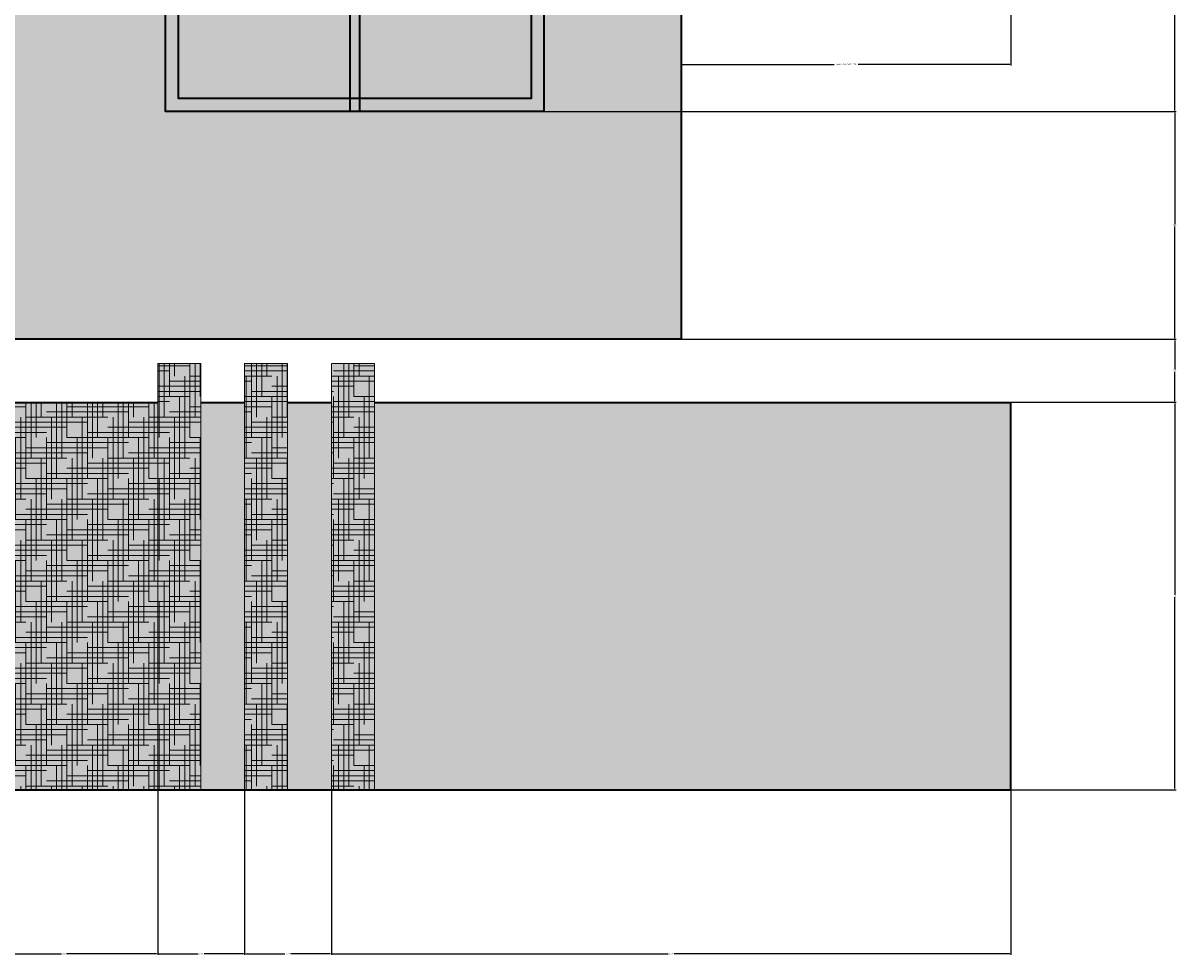
# Model space of a CAD drawing. Units: feet. Extents: x 2415 to 6174, y 866 to 1295.
# Tile 4 of 9: x 3580 to 3759, y 866 to 1010. Entities that reach past the tile are written whole.
import ezdxf

# ---------------------------------------------------------------- set-up
doc = ezdxf.new("R2010")
doc.units = ezdxf.units.FT
for name, color, linetype, lineweight in [('A-ANNO-DIMS', 2, 'Continuous', 18), ('A-ELEV', 7, 'Continuous', 35), ('A-ELEV-LOUV', 9, 'Continuous', 18), ('A-ELEV-PATT', 8, 'Continuous', 13)]:
    doc.layers.add(name, color=color, linetype=linetype, lineweight=lineweight)
doc.styles.get("Standard").update_dxf_attribs({"font": 'arial.ttf'})
doc.dimstyles.get("Standard").update_dxf_attribs({"dimtxt": 0.18, "dimasz": 0.18, "dimexe": 0.18, "dimexo": 0.0625, "dimgap": 0.09, "dimtad": 0, "dimtih": 1, "dimtoh": 1, "dimdec": 1, "dimzin": 0, "dimdsep": 46, "dimlunit": 3, "dimtxsty": 'Standard', "dimcen": 0.09, "dimadec": 0, "dimazin": 0, "dimtfac": 1, "dimtdec": 1, "dimtofl": 0, "dimtmove": 0, "dimatfit": 3, "dimfxl": 1, "dimtolj": 1, "dimtzin": 0, "dimarcsym": 0})

# ---------------------------------------------------------------- blocks, each defined once
blk = doc.blocks.new('FACADE-FIN')
blk.add_line((0, 66), (6.66, 66))
for points in [[(0, 0), (0, 66)], [(6.66, 66), (6.66, 0)]]:
    blk.add_lwpolyline(points)
blk = doc.blocks.new('*D13')
at = {"layer": 'A-ANNO-DIMS', "color": 0, "lineweight": -2, "transparency": 16777216}
for p, q in [((3682.07, 1011.54), (3682.07, 1003.76)), ((3733.13, 1011.54), (3733.13, 1003.76)), ((3682.25, 1003.94), (3705.76, 1003.94)), ((3732.95, 1003.94), (3709.45, 1003.94))]:
    blk.add_line(p, q, dxfattribs=at)
at = {"layer": 'A-ANNO-DIMS', "color": 0, "transparency": 16777216}
for points in [[(3682.25, 1003.97), (3682.25, 1003.91), (3682.07, 1003.94)], [(3732.95, 1003.97), (3732.95, 1003.91), (3733.13, 1003.94)]]:
    blk.add_solid(points, dxfattribs=at)
at = {"layer": 'Defpoints', "color": 0, "transparency": 16777216}
for p in [(3682.07, 1011.6), (3733.13, 1011.6), (3733.13, 1003.94)]:
    blk.add_point(p, dxfattribs=at)
at = {"layer": 'A-ANNO-DIMS', "color": 0, "transparency": 16777216, "insert": (3707.6, 1003.94), "char_height": 0.18, "attachment_point": 5}
blk.add_mtext('\\A1;BALCONY RAIL BASE 51 TYP.', dxfattribs=at)
blk = doc.blocks.new('*D57')
at = {"layer": 'A-ANNO-DIMS', "color": 0, "lineweight": -2, "transparency": 16777216}
for p, q in [((3571.93, 891.54), (3571.93, 866.02)), ((3601, 891.54), (3601, 866.02)), ((3572.11, 866.2), (3586.07, 866.2)), ((3600.82, 866.2), (3586.86, 866.2))]:
    blk.add_line(p, q, dxfattribs=at)
at = {"layer": 'A-ANNO-DIMS', "color": 0, "transparency": 16777216}
for points in [[(3572.11, 866.23), (3572.11, 866.17), (3571.93, 866.2)], [(3600.82, 866.23), (3600.82, 866.17), (3601, 866.2)]]:
    blk.add_solid(points, dxfattribs=at)
at = {"layer": 'Defpoints', "color": 0, "transparency": 16777216}
for p in [(3571.93, 891.6), (3601, 891.6), (3601, 866.2)]:
    blk.add_point(p, dxfattribs=at)
at = {"layer": 'A-ANNO-DIMS', "color": 0, "transparency": 16777216, "insert": (3586.47, 866.2), "char_height": 0.18, "attachment_point": 5}
blk.add_mtext('\\A1;29.06', dxfattribs=at)
blk = doc.blocks.new('*D58')
at = {"layer": 'A-ANNO-DIMS', "color": 0, "lineweight": -2, "transparency": 16777216}
for p, q in [((3601, 891.54), (3601, 866.02)), ((3614.44, 891.54), (3614.44, 866.02)), ((3601.18, 866.2), (3607.26, 866.2)), ((3614.26, 866.2), (3608.17, 866.2))]:
    blk.add_line(p, q, dxfattribs=at)
at = {"layer": 'A-ANNO-DIMS', "color": 0, "transparency": 16777216}
for points in [[(3601.18, 866.23), (3601.18, 866.17), (3601, 866.2)], [(3614.26, 866.23), (3614.26, 866.17), (3614.44, 866.2)]]:
    blk.add_solid(points, dxfattribs=at)
at = {"layer": 'Defpoints', "color": 0, "transparency": 16777216}
for p in [(3601, 891.6), (3614.44, 891.6), (3614.44, 866.2)]:
    blk.add_point(p, dxfattribs=at)
at = {"layer": 'A-ANNO-DIMS', "color": 0, "transparency": 16777216, "insert": (3607.72, 866.2), "char_height": 0.18, "attachment_point": 5}
blk.add_mtext('\\A1;13.442', dxfattribs=at)
blk = doc.blocks.new('*D59')
at = {"layer": 'A-ANNO-DIMS', "color": 0, "lineweight": -2, "transparency": 16777216}
for p, q in [((3614.44, 891.54), (3614.44, 866.02)), ((3627.88, 891.54), (3627.88, 866.02)), ((3614.62, 866.2), (3620.7, 866.2)), ((3627.7, 866.2), (3621.61, 866.2))]:
    blk.add_line(p, q, dxfattribs=at)
at = {"layer": 'A-ANNO-DIMS', "color": 0, "transparency": 16777216}
for points in [[(3614.62, 866.23), (3614.62, 866.17), (3614.44, 866.2)], [(3627.7, 866.23), (3627.7, 866.17), (3627.88, 866.2)]]:
    blk.add_solid(points, dxfattribs=at)
at = {"layer": 'Defpoints', "color": 0, "transparency": 16777216}
for p in [(3614.44, 891.6), (3627.88, 891.6), (3627.88, 866.2)]:
    blk.add_point(p, dxfattribs=at)
at = {"layer": 'A-ANNO-DIMS', "color": 0, "transparency": 16777216, "insert": (3621.16, 866.2), "char_height": 0.18, "attachment_point": 5}
blk.add_mtext('\\A1;13.442', dxfattribs=at)
blk = doc.blocks.new('*D60')
at = {"layer": 'A-ANNO-DIMS', "color": 0, "lineweight": -2, "transparency": 16777216}
for p, q in [((3627.88, 891.54), (3627.88, 866.02)), ((3733.13, 891.54), (3733.13, 866.02)), ((3628.06, 866.2), (3680.05, 866.2)), ((3732.95, 866.2), (3680.96, 866.2))]:
    blk.add_line(p, q, dxfattribs=at)
at = {"layer": 'A-ANNO-DIMS', "color": 0, "transparency": 16777216}
for points in [[(3628.06, 866.23), (3628.06, 866.17), (3627.88, 866.2)], [(3732.95, 866.23), (3732.95, 866.17), (3733.13, 866.2)]]:
    blk.add_solid(points, dxfattribs=at)
at = {"layer": 'Defpoints', "color": 0, "transparency": 16777216}
for p in [(3627.88, 891.6), (3733.13, 891.6), (3733.13, 866.2)]:
    blk.add_point(p, dxfattribs=at)
at = {"layer": 'A-ANNO-DIMS', "color": 0, "transparency": 16777216, "insert": (3680.5, 866.2), "char_height": 0.18, "attachment_point": 5}
blk.add_mtext('\\A1;105.25', dxfattribs=at)
blk = doc.blocks.new('*D79')
at = {"layer": 'A-ANNO-DIMS', "color": 0, "lineweight": -2, "transparency": 16777216}
for p, q in [((3733.19, 951.6), (3758.71, 951.6)), ((3758.53, 951.42), (3758.53, 921.78)), ((3758.53, 891.78), (3758.53, 921.42)), ((3733.19, 891.6), (3758.71, 891.6))]:
    blk.add_line(p, q, dxfattribs=at)
at = {"layer": 'A-ANNO-DIMS', "color": 0, "transparency": 16777216}
for points in [[(3758.5, 951.42), (3758.56, 951.42), (3758.53, 951.6)], [(3758.5, 891.78), (3758.56, 891.78), (3758.53, 891.6)]]:
    blk.add_solid(points, dxfattribs=at)
at = {"layer": 'Defpoints', "color": 0, "transparency": 16777216}
for p in [(3733.13, 951.6), (3758.53, 951.6), (3733.13, 891.6)]:
    blk.add_point(p, dxfattribs=at)
at = {"layer": 'A-ANNO-DIMS', "color": 0, "transparency": 16777216, "insert": (3758.53, 921.6), "char_height": 0.18, "attachment_point": 5}
blk.add_mtext('\\A1;60', dxfattribs=at)
blk = doc.blocks.new('*D80')
at = {"layer": 'A-ANNO-DIMS', "color": 0, "lineweight": -2, "transparency": 16777216}
for p, q in [((3682.13, 961.37), (3758.71, 961.37)), ((3758.53, 961.19), (3758.53, 956.66)), ((3758.53, 951.78), (3758.53, 956.3)), ((3733.19, 951.6), (3758.71, 951.6))]:
    blk.add_line(p, q, dxfattribs=at)
at = {"layer": 'A-ANNO-DIMS', "color": 0, "transparency": 16777216}
for points in [[(3758.5, 961.19), (3758.56, 961.19), (3758.53, 961.37)], [(3758.5, 951.78), (3758.56, 951.78), (3758.53, 951.6)]]:
    blk.add_solid(points, dxfattribs=at)
at = {"layer": 'Defpoints', "color": 0, "transparency": 16777216}
for p in [(3682.07, 961.37), (3758.53, 961.37), (3733.13, 951.6)]:
    blk.add_point(p, dxfattribs=at)
at = {"layer": 'A-ANNO-DIMS', "color": 0, "transparency": 16777216, "insert": (3758.53, 956.48), "char_height": 0.18, "attachment_point": 5}
blk.add_mtext('\\A1;9.766', dxfattribs=at)
blk = doc.blocks.new('*D81')
at = {"layer": 'A-ANNO-DIMS', "color": 0, "lineweight": -2, "transparency": 16777216}
for p, q in [((3660.88, 996.64), (3758.71, 996.64)), ((3758.53, 996.46), (3758.53, 979.19)), ((3758.53, 961.55), (3758.53, 978.82)), ((3682.13, 961.37), (3758.71, 961.37))]:
    blk.add_line(p, q, dxfattribs=at)
at = {"layer": 'A-ANNO-DIMS', "color": 0, "transparency": 16777216}
for points in [[(3758.5, 996.46), (3758.56, 996.46), (3758.53, 996.64)], [(3758.5, 961.55), (3758.56, 961.55), (3758.53, 961.37)]]:
    blk.add_solid(points, dxfattribs=at)
at = {"layer": 'Defpoints', "color": 0, "transparency": 16777216}
for p in [(3660.81, 996.64), (3758.53, 996.64), (3682.07, 961.37)]:
    blk.add_point(p, dxfattribs=at)
at = {"layer": 'A-ANNO-DIMS', "color": 0, "transparency": 16777216, "insert": (3758.53, 979.01), "char_height": 0.18, "attachment_point": 5}
blk.add_mtext('\\A1;35.28', dxfattribs=at)
blk = doc.blocks.new('*D82')
at = {"layer": 'A-ANNO-DIMS', "color": 0, "lineweight": -2, "transparency": 16777216}
for p, q in [((3660.88, 1029.3), (3758.71, 1029.3)), ((3758.53, 1029.12), (3758.53, 1013.16)), ((3758.53, 996.82), (3758.53, 1012.79)), ((3660.88, 996.64), (3758.71, 996.64))]:
    blk.add_line(p, q, dxfattribs=at)
at = {"layer": 'A-ANNO-DIMS', "color": 0, "transparency": 16777216}
for points in [[(3758.5, 1029.12), (3758.56, 1029.12), (3758.53, 1029.3)], [(3758.5, 996.82), (3758.56, 996.82), (3758.53, 996.64)]]:
    blk.add_solid(points, dxfattribs=at)
at = {"layer": 'Defpoints', "color": 0, "transparency": 16777216}
for p in [(3660.81, 1029.3), (3758.53, 1029.3), (3660.81, 996.64)]:
    blk.add_point(p, dxfattribs=at)
at = {"layer": 'A-ANNO-DIMS', "color": 0, "transparency": 16777216, "insert": (3758.53, 1012.97), "char_height": 0.18, "attachment_point": 5}
blk.add_mtext('\\A1;32.66', dxfattribs=at)

msp = doc.modelspace()

# ---------------------------------------------------------------- hatches: boundary and pattern name
at = {"layer": 'A-ELEV-PATT'}
h = msp.add_hatch(color=256, dxfattribs=at)
h.set_gradient(color1=(255, 255, 255), tint=1)
h.paths.add_polyline_path([(3264.916, 1143.5993), (3253.129, 1143.5993), (3253.129, 891.5992), (3264.916, 891.5992)])
h.paths.add_polyline_path([(3470.0448, 1143.5993), (3264.916, 1143.5993), (3264.916, 1137.5993), (3466.5999, 1137.5993)])
h.paths.add_polyline_path([(3363.8667, 1137.5993), (3264.916, 1137.5993), (3264.916, 1011.5993), (3363.8667, 1011.5993)])
h.paths.add_polyline_path([(3286.0429, 1117.0591), (3337.7904, 1117.0591), (3337.7904, 1115.4381), (3336.5314, 1115.4381), (3336.5314, 1110.528), (3335.4882, 1110.528), (3335.4882, 1042.3194), (3288.3452, 1042.3194), (3288.3452, 1110.528), (3287.3019, 1110.528), (3287.3019, 1115.4381), (3286.0429, 1115.4381)], flags=16)
h.paths.add_polyline_path([(3290.3452, 1108.528), (3333.4882, 1108.528), (3333.4882, 1044.3194), (3290.3452, 1044.3194)], flags=0)
h.paths.add_polyline_path([(3292.3452, 1106.528), (3331.4882, 1106.528), (3331.4882, 1046.3194), (3292.3452, 1046.3194)], flags=0)
h.paths.add_polyline_path([(3311.7156, 1106.528), (3312.1178, 1106.528), (3312.1178, 1046.3194), (3311.7156, 1046.3194)], flags=0)
h.paths.add_polyline_path([(3682.0722, 1263.5993), (3578.5579, 1263.5993), (3578.5579, 1137.5993), (3578.5579, 961.3655), (3682.0722, 961.3655)])
h.paths.add_polyline_path([(3660.8129, 1239.0671), (3660.8129, 996.6447), (3602.2151, 996.6447), (3602.2151, 1239.0671)], flags=16)
h.paths.add_polyline_path([(3632.2447, 1239.0671), (3632.2447, 996.6447), (3630.7833, 996.6447), (3630.7833, 1029.3019), (3602.2151, 1029.3019), (3602.2151, 1030.7632), (3630.7833, 1030.7632), (3630.7833, 1071.2549), (3602.2151, 1071.2549), (3602.2151, 1072.7163), (3630.7833, 1072.7163), (3630.7833, 1113.2079), (3602.2151, 1113.2079), (3602.2151, 1114.6693), (3630.7833, 1114.6693), (3630.7833, 1155.161), (3602.2151, 1155.161), (3602.2151, 1156.6224), (3630.7833, 1156.6224), (3630.7833, 1197.114), (3602.2151, 1197.114), (3602.2151, 1198.5754), (3630.7833, 1198.5754), (3630.7833, 1239.0671)], flags=0)
h.paths.add_polyline_path([(3733.129, 951.5992), (3634.5374, 951.5992), (3634.5374, 891.5992), (3733.129, 891.5992)])
h.paths.add_polyline_path([(3627.8799, 951.5992), (3621.0953, 951.5992), (3621.0953, 891.5992), (3627.8799, 891.5992)])
h.paths.add_polyline_path([(3614.4378, 951.5992), (3607.6532, 951.5992), (3607.6532, 891.5992), (3614.4378, 891.5992)])
h.paths.add_polyline_path([(3565.9347, 951.5992), (3441.3079, 951.5992), (3441.3079, 891.5992), (3565.9347, 891.5992)], flags=17)
h.paths.add_polyline_path([(3571.9347, 957.5993), (3435.3079, 957.5993), (3435.3079, 891.5992), (3441.3079, 891.5992), (3441.3079, 951.5992), (3565.9347, 951.5992), (3565.9347, 891.5992), (3571.9347, 891.5992)])
h.paths.add_polyline_path([(3435.3079, 1011.5993), (3423.5209, 1011.5993), (3423.5209, 891.5992), (3435.3079, 891.5992), (3435.3079, 957.5993)])
h.paths.add_polyline_path([(3690.0912, 1269.5993), (3571.9347, 1269.5993), (3571.9347, 1263.5993), (3690.0912, 1263.5993)])
h.paths.add_polyline_path([(3571.9347, 1269.5993), (3538.5122, 1257.6449), (3538.5122, 1251.6449), (3571.9347, 1263.5993)])
h = msp.add_hatch(color=256, dxfattribs=at)
h.set_gradient(color1=(99, 100, 102), color2=(99, 100, 102))
h.paths.add_polyline_path([(3660.8129, 1239.0671), (3602.2151, 1239.0671), (3602.2151, 996.6447), (3660.8129, 996.6447)])
h.paths.add_polyline_path([(3604.2151, 1237.0671), (3658.8129, 1237.0671), (3658.8129, 998.6447), (3604.2151, 998.6447)], flags=16)
h = msp.add_hatch(color=256, dxfattribs=at)
h.set_gradient(color1=(181, 210, 237), color2=(122, 175, 223))
h.paths.add_polyline_path([(3630.7833, 1239.0671), (3602.2151, 1239.0671), (3602.2151, 1198.5754), (3630.7833, 1198.5754)])
h.paths.add_polyline_path([(3660.8129, 1239.0671), (3632.2447, 1239.0671), (3632.2447, 1198.5754), (3660.8129, 1198.5754)])
h.paths.add_polyline_path([(3630.7833, 1197.114), (3602.2151, 1197.114), (3602.2151, 1156.6224), (3630.7833, 1156.6224)])
h.paths.add_polyline_path([(3660.8129, 1197.114), (3632.2447, 1197.114), (3632.2447, 1156.6224), (3660.8129, 1156.6224)])
h.paths.add_polyline_path([(3630.7833, 1155.161), (3602.2151, 1155.161), (3602.2151, 1114.6693), (3630.7833, 1114.6693)])
h.paths.add_polyline_path([(3660.8129, 1155.161), (3632.2447, 1155.161), (3632.2447, 1114.6693), (3660.8129, 1114.6693)])
h.paths.add_polyline_path([(3630.7833, 1113.2079), (3602.2151, 1113.2079), (3602.2151, 1072.7163), (3630.7833, 1072.7163)])
h.paths.add_polyline_path([(3660.8129, 1113.2079), (3632.2447, 1113.2079), (3632.2447, 1072.7163), (3660.8129, 1072.7163)])
h.paths.add_polyline_path([(3660.8129, 1071.2549), (3632.2447, 1071.2549), (3632.2447, 996.6447), (3660.8129, 996.6447)])
h.paths.add_polyline_path([(3630.7833, 1071.2549), (3602.2151, 1071.2549), (3602.2151, 1030.7632), (3630.7833, 1030.7632)])
h.paths.add_polyline_path([(3630.7833, 1029.3019), (3602.2151, 1029.3019), (3602.2151, 996.6447), (3630.7833, 996.6447)])
h = msp.add_hatch(color=256, dxfattribs=at)
h.set_gradient(color2=(0, 0, 0))
h.paths.add_polyline_path([(3630.7833, 1030.7632), (3604.2151, 1030.7632), (3604.2151, 1029.3019), (3630.7833, 1029.3019)])
h.paths.add_polyline_path([(3658.8129, 1030.7632), (3632.2447, 1030.7632), (3632.2447, 1029.3019), (3658.8129, 1029.3019)])
h.paths.add_polyline_path([(3632.2447, 1030.7632), (3630.7833, 1030.7632), (3630.7833, 1029.3019), (3632.2447, 1029.3019)])
h.paths.add_polyline_path([(3632.2447, 1239.0671), (3630.7833, 1239.0671), (3630.7833, 1030.7632), (3632.2447, 1030.7632)])
h.paths.add_polyline_path([(3632.2447, 1029.3019), (3630.7833, 1029.3019), (3630.7833, 996.6447), (3632.2447, 996.6447)])
h = msp.add_hatch(color=256, dxfattribs=at)
h.set_gradient(color1=(99, 100, 102), color2=(99, 100, 102))
h.paths.add_polyline_path([(3607.6532, 957.5993), (3600.9957, 957.5993), (3600.9957, 891.5992), (3607.6532, 891.5992)])
h.paths.add_polyline_path([(3621.0953, 957.5993), (3614.4378, 957.5993), (3614.4378, 891.5992), (3621.0953, 891.5992)])
h.paths.add_polyline_path([(3634.5374, 957.5993), (3627.8799, 957.5993), (3627.8799, 891.5992), (3634.5374, 891.5992)])
h.paths.add_polyline_path([(3600.9957, 951.5992), (3571.9347, 951.5992), (3571.9347, 891.5992), (3600.9957, 891.5992)])
h = msp.add_hatch(dxfattribs=at)
h.set_pattern_fill('HOUND', color=256, scale=0.5, style=0)
h.set_pattern_definition([(0, (850.0754, 0), (3.175, 0.79375), [12.7, -6.35]), (90, (850.0754, 0), (-0.79375, -3.175), [12.7, -6.35])])
h.paths.add_polyline_path([(3607.6532, 957.5993), (3600.9957, 957.5993), (3600.9957, 891.5992), (3607.6532, 891.5992)])
h.paths.add_polyline_path([(3621.0953, 957.5993), (3614.4378, 957.5993), (3614.4378, 891.5992), (3621.0953, 891.5992)])
h.paths.add_polyline_path([(3634.5374, 957.5993), (3627.8799, 957.5993), (3627.8799, 891.5992), (3634.5374, 891.5992)])
h.paths.add_polyline_path([(3600.9957, 951.5992), (3571.9347, 951.5992), (3571.9347, 891.5992), (3600.9957, 891.5992)])

# ---------------------------------------------------------------- linework, layer by layer
at = {"layer": 'A-ELEV'}
for p, q in [((3571.9347, 951.5992), (3600.9957, 951.5992)), ((3607.6532, 951.5992), (3614.4378, 951.5992)), ((3621.0953, 951.5992), (3627.8799, 951.5992)), ((3634.5374, 951.5992), (3733.129, 951.5992)), ((3733.129, 891.5992), (3733.129, 951.5992)), ((3253.129, 891.5992), (3733.129, 891.5992))]:
    msp.add_line(p, q, dxfattribs=at)
msp.add_lwpolyline([(3682.0722, 1263.5993), (3682.0722, 961.3655), (3578.5579, 961.3655)], dxfattribs=at)
for points in [[(3602.2151, 1239.0671), (3660.8129, 1239.0671), (3660.8129, 996.6447), (3602.2151, 996.6447)], [(3630.7833, 1239.0671), (3632.2447, 1239.0671), (3632.2447, 996.6447), (3630.7833, 996.6447)], [(3604.2151, 1237.0671), (3658.8129, 1237.0671), (3658.8129, 998.6447), (3604.2151, 998.6447)]]:
    msp.add_lwpolyline(points, close=True, dxfattribs=at)

# ---------------------------------------------------------------- block references
at = {"layer": 'A-ELEV-LOUV'}
for p in [(3600.9958, 891.599), (3614.4379, 891.599), (3627.88, 891.599)]:
    msp.add_blockref('FACADE-FIN', p, dxfattribs=at)

# ---------------------------------------------------------------- dimensions: what is measured, and where the dimension line sits
at = {"layer": 'A-ANNO-DIMS'}
for base, p1, p2, override, picture, middle in [((3758.529, 1029.3019), (3660.8129, 996.6447), (3660.8129, 1029.3019), {"dimdec": 2, "dimlfac": 1, "dimrnd": 0, "dimzin": 0, "dimdsep": 46, "dimlunit": 2}, '*D82', (3758.529, 1012.9733)), ((3758.529, 996.6447), (3682.0722, 961.3655), (3660.8129, 996.6447), {"dimdec": 2, "dimlfac": 1, "dimrnd": 0, "dimzin": 0, "dimdsep": 46, "dimlunit": 2}, '*D81', (3758.529, 979.0051)), ((3758.529, 961.3655), (3733.129, 951.5992), (3682.0722, 961.3655), {"dimdec": 3, "dimlfac": 1, "dimrnd": 0, "dimzin": 0, "dimdsep": 46, "dimlunit": 2}, '*D80', (3758.529, 956.4824)), ((3758.529, 951.5992), (3733.129, 891.5992), (3733.129, 951.5992), {"dimdec": 0, "dimlfac": 1, "dimrnd": 0, "dimzin": 0, "dimdsep": 46, "dimlunit": 2}, '*D79', (3758.529, 921.5992))]:
    dim = msp.add_linear_dim(base=base, p1=p1, p2=p2, angle=90, dimstyle='Standard', override=override, dxfattribs=at)
    dim.commit()
    dim.dimension.update_dxf_attribs({"geometry": picture, "text_midpoint": middle})
dim = msp.add_linear_dim(base=(3733.129, 1003.9407), p1=(3682.0722, 1011.5993), p2=(3733.129, 1011.5993), text='BALCONY RAIL BASE <> TYP.', dimstyle='Standard', override={"dimdec": 0, "dimrnd": 0, "dimzin": 0, "dimlunit": 2}, dxfattribs=at)
dim.commit()
dim.dimension.update_dxf_attribs({"geometry": '*D13', "text_midpoint": (3707.6006, 1003.9407)})
for base, p1, p2, override, picture, middle in [((3600.9957, 866.1993), (3571.9347, 891.5992), (3600.9957, 891.5992), {"dimdec": 2, "dimlfac": 1, "dimrnd": 0, "dimzin": 0, "dimdsep": 46, "dimlunit": 2}, '*D57', (3586.4652, 866.1993)), ((3614.4378, 866.1993), (3600.9957, 891.5992), (3614.4378, 891.5992), {"dimdec": 3, "dimlfac": 1, "dimrnd": 0, "dimzin": 0, "dimdsep": 46, "dimlunit": 2}, '*D58', (3607.7168, 866.1993)), ((3627.8799, 866.1993), (3614.4378, 891.5992), (3627.8799, 891.5992), {"dimdec": 3, "dimlfac": 1, "dimrnd": 0, "dimzin": 0, "dimdsep": 46, "dimlunit": 2}, '*D59', (3621.1589, 866.1993)), ((3733.129, 866.1993), (3627.8799, 891.5992), (3733.129, 891.5992), {"dimdec": 2, "dimlfac": 1, "dimrnd": 0, "dimzin": 0, "dimdsep": 46, "dimlunit": 2}, '*D60', (3680.5044, 866.1993))]:
    dim = msp.add_linear_dim(base=base, p1=p1, p2=p2, dimstyle='Standard', override=override, dxfattribs=at)
    dim.commit()
    dim.dimension.update_dxf_attribs({"geometry": picture, "text_midpoint": middle})

doc.saveas('drawing.dxf')
